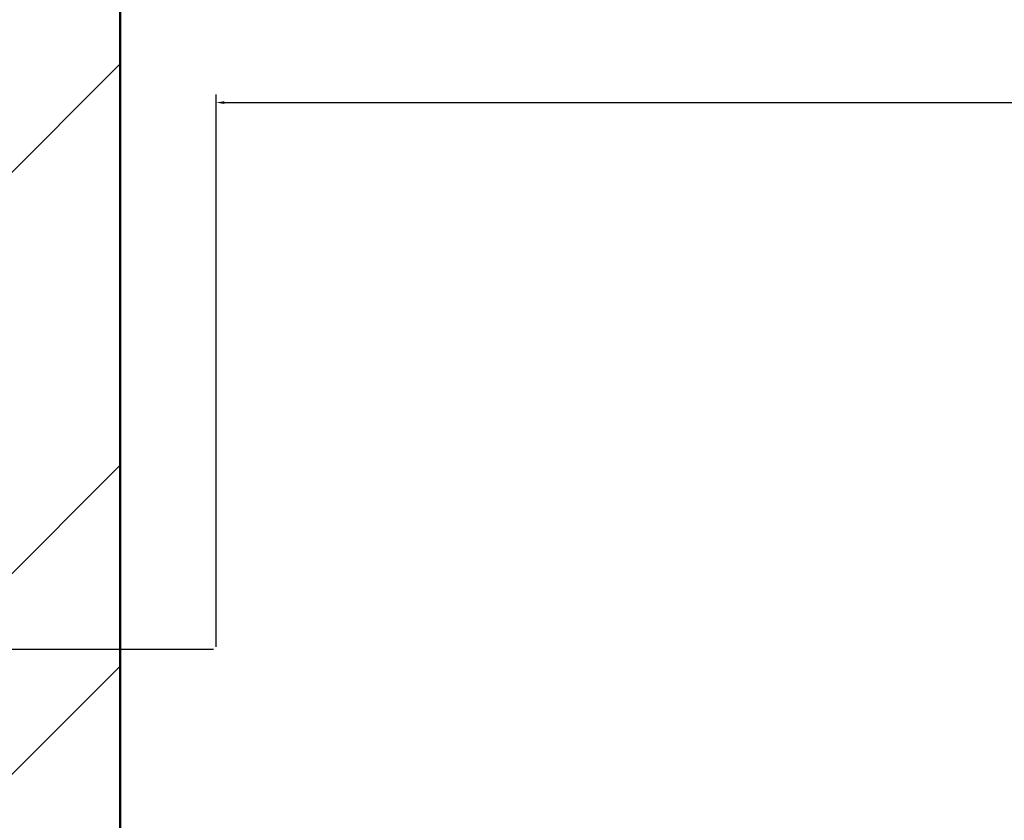
# Model space of a CAD drawing. Units: inches. Extents: x 963 to 2075, y 289 to 2657.
# Tile 40 of 98: x 1511 to 1533, y 1640 to 1658. Entities that reach past the tile are written whole.
import ezdxf

# ---------------------------------------------------------------- set-up
doc = ezdxf.new("R2010")
doc.units = ezdxf.units.IN
for name, color, linetype, lineweight in [('A-ANNO-DIMS', 2, 'Continuous', 18), ('A-WALL', 7, 'Continuous', 50), ('A-WALL-PATT', 8, 'Continuous', 13)]:
    doc.layers.add(name, color=color, linetype=linetype, lineweight=lineweight)
doc.styles.get("Standard").update_dxf_attribs({"font": 'arial.ttf'})
doc.dimstyles.get("Standard").update_dxf_attribs({"dimtxt": 0.18, "dimasz": 0.18, "dimexe": 0.18, "dimexo": 0.0625, "dimgap": 0.09, "dimtad": 0, "dimtih": 1, "dimtoh": 1, "dimdec": 4, "dimzin": 0, "dimdsep": 46, "dimtxsty": 'Standard', "dimcen": 0.09, "dimadec": 0, "dimazin": 0, "dimtfac": 1, "dimtdec": 4, "dimtofl": 0, "dimtmove": 0, "dimatfit": 3, "dimfxl": 1, "dimtolj": 1, "dimtzin": 0, "dimarcsym": 0})

# ---------------------------------------------------------------- blocks, each defined once
blk = doc.blocks.new('*D14')
at = {"layer": 'A-ANNO-DIMS', "color": 0, "lineweight": -2, "transparency": 16777216}
for p, q in [((1515.065, 1643.568), (1515.065, 1655.918)), ((1596.614, 1643.568), (1596.614, 1655.918)), ((1515.245, 1655.738), (1554.47, 1655.738)), ((1596.434, 1655.738), (1557.208, 1655.738))]:
    blk.add_line(p, q, dxfattribs=at)
at = {"layer": 'A-ANNO-DIMS', "color": 0, "transparency": 16777216}
for points in [[(1515.245, 1655.768), (1515.245, 1655.708), (1515.065, 1655.738)], [(1596.434, 1655.768), (1596.434, 1655.708), (1596.614, 1655.738)]]:
    blk.add_solid(points, dxfattribs=at)
at = {"layer": 'Defpoints', "color": 0, "transparency": 16777216}
for p in [(1515.065, 1655.738), (1515.065, 1643.505), (1596.614, 1643.505)]:
    blk.add_point(p, dxfattribs=at)
at = {"layer": 'A-ANNO-DIMS', "color": 0, "transparency": 16777216, "insert": (1555.839, 1655.738), "char_height": 0.18, "attachment_point": 5}
blk.add_mtext('\\A1;DOUBLE BED 82 TYP.', dxfattribs=at)
blk = doc.blocks.new('*D15')
at = {"layer": 'A-ANNO-DIMS', "color": 0, "lineweight": -2, "transparency": 16777216}
for p, q in [((1515.003, 1643.505), (1502.653, 1643.505)), ((1502.833, 1643.325), (1502.833, 1615.775)), ((1502.833, 1587.861), (1502.833, 1615.411)), ((1515.003, 1587.681), (1502.653, 1587.681))]:
    blk.add_line(p, q, dxfattribs=at)
at = {"layer": 'A-ANNO-DIMS', "color": 0, "transparency": 16777216}
for points in [[(1502.803, 1643.325), (1502.863, 1643.325), (1502.833, 1643.505)], [(1502.803, 1587.861), (1502.863, 1587.861), (1502.833, 1587.681)]]:
    blk.add_solid(points, dxfattribs=at)
at = {"layer": 'Defpoints', "color": 0, "transparency": 16777216}
for p in [(1515.065, 1643.505), (1502.833, 1587.681), (1515.065, 1587.681)]:
    blk.add_point(p, dxfattribs=at)
at = {"layer": 'A-ANNO-DIMS', "color": 0, "transparency": 16777216, "insert": (1502.833, 1615.593), "char_height": 0.18, "attachment_point": 5}
blk.add_mtext('\\A1;56 TYP.', dxfattribs=at)

msp = doc.modelspace()

# ---------------------------------------------------------------- hatches: boundary and pattern name
at = {"layer": 'A-WALL-PATT'}
h = msp.add_hatch(dxfattribs=at)
h.set_pattern_fill('ANSI32', color=256)
h.paths.add_polyline_path([(1473.609, 2163.068), (1473.609, 2165.318), (1376.422, 2165.318), (1376.422, 2227.983), (1371.922, 2227.983), (1371.922, 2214.818), (1368.405, 2214.818), (1368.405, 2210.318), (1371.922, 2210.318), (1371.922, 2160.818), (1395.922, 2160.818), (1395.922, 2090.318), (1217.345, 2090.318), (1217.345, 2085.818), (1395.922, 2085.818), (1458.922, 2085.818), (1458.922, 2108.318), (1454.422, 2108.318), (1454.422, 2090.318), (1400.422, 2090.318), (1400.422, 2160.818), (1473.609, 2160.818)])
h.paths.add_polyline_path([(1649.422, 2210.318), (1653.225, 2210.318), (1653.225, 2214.818), (1649.422, 2214.818), (1649.422, 2227.983), (1644.922, 2227.983), (1644.922, 2165.318), (1550.099, 2165.318), (1550.099, 2160.818), (1620.922, 2160.818), (1620.922, 2112.818), (1555.446, 2112.818), (1555.446, 2108.318), (1584.327, 2108.318), (1584.327, 2084.916), (1588.827, 2084.916), (1588.827, 2108.318), (1625.422, 2108.318), (1667.951, 2108.318), (1667.951, 2022.667), (1588.827, 2022.667), (1588.827, 2047.408), (1584.327, 2047.408), (1584.327, 1996.003), (1588.827, 1996.003), (1588.827, 2018.318), (1667.951, 2018.167), (1667.951, 1928.318), (1625.422, 1928.318), (1625.422, 1923.818), (1672.451, 1923.818), (1672.451, 1928.318), (1672.451, 1946.663), (1785.446, 1946.663), (1785.446, 1951.163), (1743.034, 1951.163), (1743.034, 2017.922), (1841.422, 2017.922), (1841.422, 2014.775), (1845.922, 2014.775), (1845.922, 2017.922), (1905.922, 2017.922), (1905.922, 1987.511), (1910.422, 1987.511), (1910.422, 2022.422), (1910.422, 2068.517), (1905.922, 2068.517), (1905.922, 2022.422), (1845.922, 2022.422), (1845.922, 2025.851), (1843.672, 2025.851), (1841.422, 2025.851), (1841.422, 2022.422), (1743.034, 2022.422), (1743.034, 2084.031), (1768.451, 2084.031), (1785.446, 2084.031), (1785.446, 2088.531), (1672.451, 2088.531), (1672.451, 2112.818), (1667.951, 2112.818), (1625.422, 2112.818), (1625.422, 2160.818), (1649.422, 2160.818)])
h.paths.add_polyline_path([(1672.451, 2084.031), (1738.534, 2084.031), (1738.534, 1951.163), (1672.451, 1951.163)], flags=16)
h.paths.add_polyline_path([(1672.451, 2084.031), (1738.534, 2084.031), (1705.492, 2017.597)], flags=0)
h.paths.add_polyline_path([(1262.766, 2085.818), (1258.266, 2085.818), (1258.266, 2023.278), (1184.422, 2023.278), (1184.422, 2018.778), (1258.266, 2018.778), (1258.266, 1950.818), (1262.766, 1950.818)])
h.paths.add_polyline_path([(1312.266, 2085.818), (1307.766, 2085.818), (1307.766, 1950.818), (1312.266, 1950.818)])
h.paths.add_polyline_path([(1458.922, 1950.818), (1395.922, 1950.818), (1216.568, 1950.818), (1216.568, 1946.318), (1346.422, 1946.318), (1395.922, 1946.318), (1395.922, 1875.818), (1371.922, 1875.818), (1371.922, 1826.318), (1368.931, 1826.318), (1368.931, 1821.818), (1371.922, 1821.818), (1371.922, 1813.622), (1376.422, 1813.622), (1376.422, 1871.318), (1474.504, 1871.318), (1474.504, 1873.568), (1474.504, 1875.818), (1400.422, 1875.818), (1400.422, 1946.318), (1454.422, 1946.318), (1454.422, 1928.318), (1458.922, 1928.318)])
h.paths.add_polyline_path([(1184.422, 2120.778), (1167.922, 2120.778), (1167.922, 2134.812), (1165.672, 2134.812), (1163.422, 2134.812), (1163.422, 2120.778), (1119.922, 2120.778), (1119.922, 2098.095), (1124.422, 2098.095), (1124.422, 2116.278), (1167.922, 2116.278), (1179.922, 2116.278), (1179.922, 2045.916), (1184.422, 2045.916), (1184.422, 2090.318), (1184.422, 2116.278)])
h.paths.add_polyline_path([(1124.422, 2018.778), (1179.922, 2018.778), (1179.922, 2016.294), (1184.422, 2016.294), (1184.422, 2023.278), (1184.422, 2026.588), (1182.172, 2026.588), (1179.922, 2026.588), (1179.922, 2023.278), (1124.422, 2023.278), (1124.422, 2074.095), (1119.922, 2074.095), (1119.922, 2018.778), (1119.922, 1979.633), (1124.422, 1979.633)])
h.paths.add_polyline_path([(1184.422, 1925.778), (1184.422, 1946.318), (1184.422, 1996.073), (1182.172, 1996.073), (1179.922, 1996.073), (1179.922, 1925.778), (1124.422, 1925.778), (1124.422, 1955.633), (1119.922, 1955.502), (1119.922, 1921.278), (1158.922, 1921.278), (1158.922, 1909.983), (1163.422, 1909.983), (1163.422, 1921.278), (1184.422, 1921.278)])
h.paths.add_polyline_path([(1341.449, 1826.318), (1163.422, 1826.318), (1163.422, 1849.983), (1158.922, 1849.983), (1158.922, 1821.818), (1158.922, 1804.033), (1163.422, 1804.033), (1163.422, 1821.818), (1341.449, 1821.818)])
h.paths.add_polyline_path([(1222.981, 1713.818), (1163.422, 1713.818), (1163.422, 1744.033), (1161.172, 1744.033), (1158.922, 1744.033), (1158.922, 1713.818), (1119.922, 1713.818), (1119.922, 1694.65), (1124.422, 1694.65), (1124.422, 1709.318), (1158.922, 1709.318), (1222.981, 1709.318)])
h.paths.add_polyline_path([(1328.422, 1713.818), (1252.042, 1713.818), (1252.042, 1711.568), (1252.042, 1709.318), (1256.422, 1709.318), (1256.422, 1547.318), (1232.937, 1547.318), (1232.937, 1545.068), (1232.937, 1542.818), (1292.422, 1542.818), (1292.422, 1527.634), (1296.922, 1527.634), (1296.922, 1542.818), (1299.464, 1542.818), (1299.464, 1547.318), (1260.922, 1547.318), (1260.922, 1658.318), (1343.661, 1658.318), (1343.661, 1660.568), (1343.661, 1662.818), (1328.422, 1662.818), (1328.422, 1676.589), (1327.402, 1676.589), (1323.922, 1676.589), (1323.922, 1662.818), (1260.922, 1662.818), (1260.922, 1709.318), (1323.922, 1709.318), (1323.922, 1699.851), (1328.422, 1699.851)])
h.paths.add_polyline_path([(1649.422, 1875.818), (1625.422, 1875.818), (1625.422, 1928.318), (1620.922, 1928.318), (1588.827, 1928.318), (1588.827, 1950.59), (1584.327, 1950.59), (1584.327, 1928.318), (1555.446, 1928.318), (1555.446, 1923.818), (1620.922, 1923.818), (1620.922, 1875.818), (1548.952, 1875.818), (1548.952, 1873.568), (1548.952, 1871.318), (1644.922, 1871.318), (1644.922, 1813.622), (1649.422, 1813.622), (1649.422, 1821.818), (1652.045, 1821.818), (1652.045, 1824.068), (1652.045, 1826.318), (1649.422, 1826.318)])
h.paths.add_polyline_path([(1512.922, 1871.318), (1516.476, 1871.318), (1516.476, 1875.818), (1512.922, 1875.818), (1512.922, 1923.818), (1512.922, 1928.318), (1512.922, 1930.827), (1508.422, 1930.827), (1508.422, 1875.818), (1504.411, 1875.818), (1504.411, 1871.318), (1508.422, 1871.318), (1508.422, 1713.818), (1376.422, 1713.818), (1376.422, 1743.325), (1371.922, 1743.325), (1371.922, 1709.318), (1371.922, 1706.01), (1376.422, 1706.01), (1376.422, 1709.318), (1508.422, 1709.318), (1508.422, 1547.318), (1501.871, 1547.318), (1501.871, 1542.818), (1508.422, 1542.818), (1508.422, 1482.818), (1508.422, 1436.318), (1512.922, 1436.318), (1512.922, 1542.818), (1519.318, 1542.818), (1519.318, 1545.068), (1519.318, 1547.318), (1512.922, 1547.318), (1512.922, 1709.318), (1644.922, 1709.318), (1644.922, 1707.548), (1649.422, 1707.548), (1649.422, 1709.318), (1649.422, 1743.325), (1644.922, 1743.325), (1644.922, 1713.818), (1512.922, 1713.818)])
h.paths.add_polyline_path([(1129.884, 1545.068), (1129.884, 1547.318), (1124.422, 1547.318), (1095.922, 1547.318), (1095.922, 1614.818), (1124.422, 1614.818), (1124.422, 1619.318), (1095.922, 1619.318), (1091.422, 1619.318), (1091.422, 1542.818), (1095.922, 1542.818), (1119.922, 1542.818), (1129.884, 1542.818)])
h.paths.add_polyline_path([(1208.422, 1542.818), (1211.74, 1542.818), (1211.74, 1547.318), (1198.851, 1547.318), (1198.851, 1542.818), (1203.922, 1542.818), (1203.922, 1478.318), (1208.422, 1478.318), (1296.922, 1478.318), (1296.922, 1503.634), (1292.422, 1503.634), (1292.422, 1482.818), (1208.422, 1482.818)])
h.paths.add_polyline_path([(1430.422, 1542.818), (1435.699, 1542.818), (1435.699, 1545.068), (1435.699, 1547.318), (1422.658, 1547.318), (1422.658, 1545.068), (1422.658, 1542.818), (1425.922, 1542.818), (1425.922, 1482.857), (1341.922, 1482.857), (1341.922, 1502.732), (1337.422, 1502.732), (1337.422, 1478.357), (1425.922, 1478.357), (1425.922, 1440.818), (1425.922, 1436.318), (1430.422, 1436.318)])
h.paths.add_polyline_path([(1698.482, 2004.259), (1727.695, 2004.259), (1727.695, 2022.916), (1698.482, 2022.916)], flags=8)

# ---------------------------------------------------------------- linework, layer by layer
at = {"layer": 'A-WALL'}
msp.add_line((1512.922, 1547.318), (1512.922, 1709.318), dxfattribs=at)

# ---------------------------------------------------------------- dimensions: what is measured, and where the dimension line sits
at = {"layer": 'A-ANNO-DIMS'}
for base, p1, p2, angle, text, picture, middle in [((1515.065, 1655.738), (1596.614, 1643.505), (1515.065, 1643.505), 180, 'DOUBLE BED <> TYP.', '*D14', (1555.839, 1655.738)), ((1502.833, 1587.681), (1515.065, 1643.505), (1515.065, 1587.681), 270, '<> TYP.', '*D15', (1502.833, 1615.593))]:
    dim = msp.add_linear_dim(base=base, p1=p1, p2=p2, angle=angle, text=text, dimstyle='Standard', override={"dimdec": 0, "dimlfac": 1, "dimrnd": 0, "dimzin": 0, "dimdsep": 46, "dimlunit": 2}, dxfattribs=at)
    dim.commit()
    dim.dimension.update_dxf_attribs({"geometry": picture, "text_midpoint": middle})

doc.saveas('drawing.dxf')
